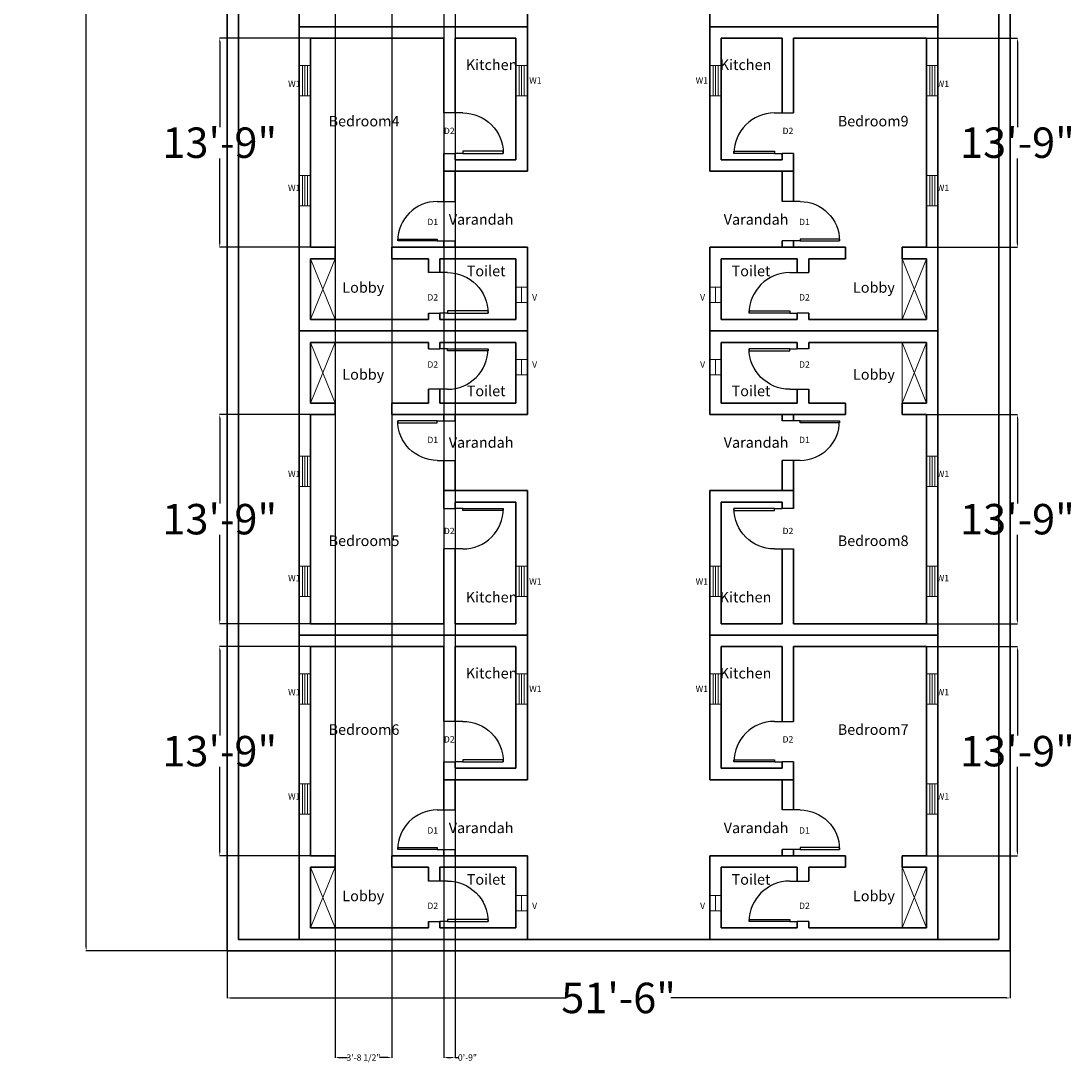
# Model space of a CAD drawing. Units: inches. Extents: x -205 to 674, y 63 to 1798.
# Tile 1 of 4: x -205 to 624, y 63 to 888. Entities that reach past the tile are written whole.
import ezdxf

# ---------------------------------------------------------------- set-up
doc = ezdxf.new("R2010")
doc.units = ezdxf.units.IN
doc.header["$MEASUREMENT"] = 0
doc.layers.get('0').update_dxf_attribs({"color": 70})
for name, color, linetype, lineweight in [('A-ANNO-DIMS', 240, 'Continuous', 18), ('A-ANNO-TEXT', 240, 'Continuous', 18), ('A-AREA-IDEN', 240, 'Continuous', 18), ('A-WALL', 70, 'Continuous', 35), ('A-WALL-SITE', 70, 'Continuous', 35), ('door1', 20, 'Continuous', 25), ('door2', 160, 'Continuous', 25), ('lobby', 241, 'Continuous', 18), ('ventilator1', 210, 'Continuous', 18), ('window1', 50, 'Continuous', 18)]:
    doc.layers.add(name, color=color, linetype=linetype, lineweight=lineweight)
doc.styles.get("Standard").update_dxf_attribs({"font": 'arial.ttf'})
doc.dimstyles.get("Standard").update_dxf_attribs({"dimtxt": 5, "dimasz": 3, "dimexe": 0.18, "dimexo": 0.0625, "dimgap": 0.09, "dimtad": 0, "dimtih": 1, "dimtoh": 1, "dimdec": 0, "dimzin": 0, "dimdsep": 46, "dimlunit": 3, "dimtxsty": 'Standard', "dimcen": 0.09, "dimadec": 0, "dimazin": 0, "dimtfac": 1, "dimtdec": 0, "dimtofl": 0, "dimtmove": 0, "dimatfit": 3, "dimfxl": 1, "dimtolj": 1, "dimtzin": 0, "dimarcsym": 0})

# ---------------------------------------------------------------- blocks, each defined once
blk = doc.blocks.new('*D8')
at = {"layer": 'A-ANNO-DIMS', "color": 0, "lineweight": -2, "transparency": 16777216}
for p, q in [((23.48, 874.3), (-48.36, 874.3)), ((-48.18, 871.3), (-48.18, 804.15)), ((-48.18, 712.3), (-48.18, 779.45)), ((23.48, 709.3), (-48.36, 709.3))]:
    blk.add_line(p, q, dxfattribs=at)
at = {"layer": 'A-ANNO-DIMS', "color": 0, "transparency": 16777216}
for points in [[(-48.68, 871.3), (-47.68, 871.3), (-48.18, 874.3)], [(-48.68, 712.3), (-47.68, 712.3), (-48.18, 709.3)]]:
    blk.add_solid(points, dxfattribs=at)
at = {"layer": 'Defpoints', "color": 0, "transparency": 16777216}
for p in [(-48.18, 874.3), (23.54, 874.3), (23.54, 709.3)]:
    blk.add_point(p, dxfattribs=at)
at = {"layer": 'A-ANNO-DIMS', "color": 0, "transparency": 16777216, "insert": (-48.18, 791.8), "char_height": 5, "attachment_point": 5}
blk.add_mtext('\\A1;{\\H4.8x;13\'-9"}', dxfattribs=at)
blk = doc.blocks.new('*U4')
for p, q in [((0, 0), (0, -6)), ((36, 0), (36, -6))]:
    blk.add_line(p, q)
blk.add_lwpolyline([(0, 0), (0, 36), (1.75, 36), (1.75, 0)], close=True)
blk.add_arc((0, 0), 36, 0, 90)
blk = doc.blocks.new('*U5')
for p, q in [((0, 0), (0, -6)), ((32, 0), (32, -6))]:
    blk.add_line(p, q)
blk.add_lwpolyline([(0, 0), (0, 32), (1.75, 32), (1.75, 0)], close=True)
blk.add_arc((0, 0), 32, 0, 90)
blk = doc.blocks.new('*D9')
at = {"layer": 'A-ANNO-DIMS', "color": 0, "lineweight": -2, "transparency": 16777216}
for p, q in [((23.48, 577.3), (-48.36, 577.3)), ((-48.18, 574.3), (-48.18, 507.15)), ((-48.18, 415.3), (-48.18, 482.45)), ((23.48, 412.3), (-48.36, 412.3))]:
    blk.add_line(p, q, dxfattribs=at)
at = {"layer": 'A-ANNO-DIMS', "color": 0, "transparency": 16777216}
for points in [[(-48.68, 574.3), (-47.68, 574.3), (-48.18, 577.3)], [(-48.68, 415.3), (-47.68, 415.3), (-48.18, 412.3)]]:
    blk.add_solid(points, dxfattribs=at)
at = {"layer": 'Defpoints', "color": 0, "transparency": 16777216}
for p in [(23.54, 577.3), (-48.18, 412.3), (23.54, 412.3)]:
    blk.add_point(p, dxfattribs=at)
at = {"layer": 'A-ANNO-DIMS', "color": 0, "transparency": 16777216, "insert": (-48.18, 494.8), "char_height": 5, "attachment_point": 5}
blk.add_mtext('\\A1;{\\H4.8x;13\'-9"}', dxfattribs=at)
blk = doc.blocks.new('*D10')
at = {"layer": 'A-ANNO-DIMS', "color": 0, "lineweight": -2, "transparency": 16777216}
for p, q in [((23.48, 394.3), (-48.36, 394.3)), ((-48.18, 391.3), (-48.18, 324.15)), ((-48.18, 232.3), (-48.18, 299.45)), ((23.48, 229.3), (-48.36, 229.3))]:
    blk.add_line(p, q, dxfattribs=at)
at = {"layer": 'A-ANNO-DIMS', "color": 0, "transparency": 16777216}
for points in [[(-48.68, 391.3), (-47.68, 391.3), (-48.18, 394.3)], [(-48.68, 232.3), (-47.68, 232.3), (-48.18, 229.3)]]:
    blk.add_solid(points, dxfattribs=at)
at = {"layer": 'Defpoints', "color": 0, "transparency": 16777216}
for p in [(-48.18, 394.3), (23.54, 394.3), (23.54, 229.3)]:
    blk.add_point(p, dxfattribs=at)
at = {"layer": 'A-ANNO-DIMS', "color": 0, "transparency": 16777216, "insert": (-48.18, 311.8), "char_height": 5, "attachment_point": 5}
blk.add_mtext('\\A1;{\\H4.8x;13\'-9"}', dxfattribs=at)
blk = doc.blocks.new('*D12')
at = {"layer": 'A-ANNO-DIMS', "color": 0, "lineweight": -2, "transparency": 16777216}
for p, q in [((509.6, 874.3), (581.44, 874.3)), ((581.26, 871.3), (581.26, 804.15)), ((581.26, 712.3), (581.26, 779.45)), ((509.6, 709.3), (581.44, 709.3))]:
    blk.add_line(p, q, dxfattribs=at)
at = {"layer": 'A-ANNO-DIMS', "color": 0, "transparency": 16777216}
for points in [[(580.76, 871.3), (581.76, 871.3), (581.26, 874.3)], [(580.76, 712.3), (581.76, 712.3), (581.26, 709.3)]]:
    blk.add_solid(points, dxfattribs=at)
at = {"layer": 'Defpoints', "color": 0, "transparency": 16777216}
for p in [(509.54, 874.3), (581.26, 874.3), (509.54, 709.3)]:
    blk.add_point(p, dxfattribs=at)
at = {"layer": 'A-ANNO-DIMS', "color": 0, "transparency": 16777216, "insert": (581.26, 791.8), "char_height": 5, "attachment_point": 5}
blk.add_mtext('\\A1;{\\H4.8x;13\'-9"}', dxfattribs=at)
blk = doc.blocks.new('*D13')
at = {"layer": 'A-ANNO-DIMS', "color": 0, "lineweight": -2, "transparency": 16777216}
for p, q in [((509.6, 577.3), (581.44, 577.3)), ((581.26, 574.3), (581.26, 507.15)), ((581.26, 415.3), (581.26, 482.45)), ((509.6, 412.3), (581.44, 412.3))]:
    blk.add_line(p, q, dxfattribs=at)
at = {"layer": 'A-ANNO-DIMS', "color": 0, "transparency": 16777216}
for points in [[(580.76, 574.3), (581.76, 574.3), (581.26, 577.3)], [(580.76, 415.3), (581.76, 415.3), (581.26, 412.3)]]:
    blk.add_solid(points, dxfattribs=at)
at = {"layer": 'Defpoints', "color": 0, "transparency": 16777216}
for p in [(509.54, 577.3), (509.54, 412.3), (581.26, 412.3)]:
    blk.add_point(p, dxfattribs=at)
at = {"layer": 'A-ANNO-DIMS', "color": 0, "transparency": 16777216, "insert": (581.26, 494.8), "char_height": 5, "attachment_point": 5}
blk.add_mtext('\\A1;{\\H4.8x;13\'-9"}', dxfattribs=at)
blk = doc.blocks.new('*D15')
at = {"layer": 'A-ANNO-DIMS', "color": 0, "lineweight": -2, "transparency": 16777216}
for p, q in [((509.6, 394.3), (581.44, 394.3)), ((581.26, 391.3), (581.26, 324.15)), ((581.26, 232.3), (581.26, 299.45)), ((509.6, 229.3), (581.44, 229.3))]:
    blk.add_line(p, q, dxfattribs=at)
at = {"layer": 'A-ANNO-DIMS', "color": 0, "transparency": 16777216}
for points in [[(580.76, 391.3), (581.76, 391.3), (581.26, 394.3)], [(580.76, 232.3), (581.76, 232.3), (581.26, 229.3)]]:
    blk.add_solid(points, dxfattribs=at)
at = {"layer": 'Defpoints', "color": 0, "transparency": 16777216}
for p in [(509.54, 394.3), (581.26, 394.3), (509.54, 229.3)]:
    blk.add_point(p, dxfattribs=at)
at = {"layer": 'A-ANNO-DIMS', "color": 0, "transparency": 16777216, "insert": (581.26, 311.8), "char_height": 5, "attachment_point": 5}
blk.add_mtext('\\A1;{\\H4.8x;13\'-9"}', dxfattribs=at)
blk = doc.blocks.new('*D18')
at = {"layer": 'A-ANNO-DIMS', "color": 0, "lineweight": -2, "transparency": 16777216}
for p, q in [((-42.52, 1660.3), (-153.74, 1660.3)), ((-153.56, 1657.3), (-153.56, 919.64)), ((-153.56, 157.3), (-153.56, 894.96)), ((-42.52, 154.3), (-153.74, 154.3))]:
    blk.add_line(p, q, dxfattribs=at)
at = {"layer": 'A-ANNO-DIMS', "color": 0, "transparency": 16777216}
for points in [[(-154.06, 1657.3), (-153.06, 1657.3), (-153.56, 1660.3)], [(-154.06, 157.3), (-153.06, 157.3), (-153.56, 154.3)]]:
    blk.add_solid(points, dxfattribs=at)
at = {"layer": 'Defpoints', "color": 0, "transparency": 16777216}
for p in [(-42.46, 1660.3), (-153.56, 154.3), (-42.46, 154.3)]:
    blk.add_point(p, dxfattribs=at)
at = {"layer": 'A-ANNO-DIMS', "color": 0, "transparency": 16777216, "insert": (-153.56, 907.3), "char_height": 5, "attachment_point": 5}
blk.add_mtext('\\A1;{\\H4.8x;125\'-6"}', dxfattribs=at)
blk = doc.blocks.new('*D19')
at = {"layer": 'A-ANNO-DIMS', "color": 0, "lineweight": -2, "transparency": 16777216}
for p, q in [((-42.46, 154.24), (-42.46, 116.92)), ((575.54, 154.24), (575.54, 116.92)), ((-39.46, 117.1), (225.23, 117.1)), ((572.54, 117.1), (307.85, 117.1))]:
    blk.add_line(p, q, dxfattribs=at)
at = {"layer": 'A-ANNO-DIMS', "color": 0, "transparency": 16777216}
for points in [[(-39.46, 117.6), (-39.46, 116.6), (-42.46, 117.1)], [(572.54, 117.6), (572.54, 116.6), (575.54, 117.1)]]:
    blk.add_solid(points, dxfattribs=at)
at = {"layer": 'Defpoints', "color": 0, "transparency": 16777216}
for p in [(-42.46, 154.3), (575.54, 154.3), (575.54, 117.1)]:
    blk.add_point(p, dxfattribs=at)
at = {"layer": 'A-ANNO-DIMS', "color": 0, "transparency": 16777216, "insert": (266.54, 117.1), "char_height": 5, "attachment_point": 5}
blk.add_mtext('\\A1;{\\H4.8x;51\'-6"}', dxfattribs=at)
blk = doc.blocks.new('WIN-W1-24IN')
for p, q in [((2.5, 24), (2.5, 0)), ((4.5, 24), (4.5, 0)), ((6.5, 24), (6.5, 0))]:
    blk.add_line(p, q)
blk.add_lwpolyline([(0, 24), (9, 24), (9, 0), (0, 0)], close=True)
blk = doc.blocks.new('VENT-V-12IN')
blk.add_line((4.5, 12), (4.5, 0))
blk.add_lwpolyline([(9, 0), (0, 0), (0, 12), (9, 12)], close=True)
blk = doc.blocks.new('LOBBY-RECESS')
for p, q in [((0, 48), (19.36, 0)), ((0, 0), (19.36, 48)), ((19.36, 48), (19.36, 0))]:
    blk.add_line(p, q)
blk = doc.blocks.new('*D40')
at = {"layer": 'A-ANNO-DIMS', "color": 0, "lineweight": -2, "transparency": 16777216}
for p, q in [((128.54, 1372.24), (128.54, 69.92)), ((137.54, 1372.24), (137.54, 69.92)), ((131.54, 70.1), (134.54, 70.1)), ((137.54, 70.1), (140.54, 70.1))]:
    blk.add_line(p, q, dxfattribs=at)
at = {"layer": 'A-ANNO-DIMS', "color": 0, "transparency": 16777216}
for points in [[(131.54, 70.6), (131.54, 69.6), (128.54, 70.1)], [(134.54, 70.6), (134.54, 69.6), (137.54, 70.1)]]:
    blk.add_solid(points, dxfattribs=at)
at = {"layer": 'Defpoints', "color": 0, "transparency": 16777216}
for p in [(128.54, 1372.3), (137.54, 1372.3), (137.54, 70.1)]:
    blk.add_point(p, dxfattribs=at)
at = {"layer": 'A-ANNO-DIMS', "color": 0, "transparency": 16777216, "insert": (147.28, 70.1), "char_height": 5, "attachment_point": 5}
blk.add_mtext('\\A1;0\'-9"', dxfattribs=at)
blk = doc.blocks.new('*D47')
at = {"layer": 'A-ANNO-DIMS', "color": 0, "lineweight": -2, "transparency": 16777216}
for p, q in [((42.9, 1546.24), (42.9, 69.92)), ((87.49, 1546.24), (87.49, 69.92)), ((45.9, 70.1), (52.64, 70.1)), ((84.49, 70.1), (77.76, 70.1))]:
    blk.add_line(p, q, dxfattribs=at)
at = {"layer": 'A-ANNO-DIMS', "color": 0, "transparency": 16777216}
for points in [[(45.9, 70.6), (45.9, 69.6), (42.9, 70.1)], [(84.49, 70.6), (84.49, 69.6), (87.49, 70.1)]]:
    blk.add_solid(points, dxfattribs=at)
at = {"layer": 'Defpoints', "color": 0, "transparency": 16777216}
for p in [(42.9, 1546.3), (87.49, 1546.3), (87.49, 70.1)]:
    blk.add_point(p, dxfattribs=at)
at = {"layer": 'A-ANNO-DIMS', "color": 0, "transparency": 16777216, "insert": (65.2, 70.1), "char_height": 5, "attachment_point": 5}
blk.add_mtext('\\A1;3\'-8 1/2"', dxfattribs=at)

msp = doc.modelspace()

# ---------------------------------------------------------------- linework, layer by layer
at = {"layer": 'A-WALL'}
for p, q in [((14.54, 883.3), (14.54, 1123.3)), ((518.54, 883.3), (518.54, 1123.3)), ((194.54, 997.3), (194.54, 883.3)), ((338.54, 997.3), (338.54, 883.3)), ((14.54, 883.3), (194.54, 883.3)), ((14.54, 883.3), (14.54, 643.3)), ((14.54, 883.3), (194.54, 883.3)), ((194.54, 769.3), (194.54, 883.3)), ((518.54, 883.3), (338.54, 883.3)), ((338.54, 769.3), (338.54, 883.3)), ((518.54, 883.3), (338.54, 883.3)), ((518.54, 883.3), (518.54, 643.3)), ((128.54, 874.3), (23.54, 874.3)), ((23.54, 874.3), (23.54, 709.3)), ((128.54, 815.3), (128.54, 874.3)), ((137.54, 815.3), (137.54, 874.3)), ((185.54, 874.3), (137.54, 874.3)), ((137.54, 815.3), (137.54, 874.3)), ((185.54, 778.3), (185.54, 874.3)), ((347.54, 778.3), (347.54, 874.3)), ((347.54, 874.3), (395.54, 874.3)), ((395.54, 815.3), (395.54, 874.3)), ((395.54, 815.3), (395.54, 874.3)), ((404.54, 815.3), (404.54, 874.3)), ((404.54, 874.3), (509.54, 874.3)), ((509.54, 874.3), (509.54, 709.3)), ((128.54, 745.41), (128.54, 783.3)), ((128.54, 783.3), (128.54, 778.3)), ((137.54, 778.3), (137.54, 783.3)), ((137.54, 778.3), (137.54, 783.3)), ((395.54, 778.3), (395.54, 783.3)), ((395.54, 778.3), (395.54, 783.3)), ((404.54, 745.41), (404.54, 783.3)), ((404.54, 783.3), (404.54, 778.3)), ((185.54, 778.3), (137.54, 778.3)), ((347.54, 778.3), (395.54, 778.3)), ((194.54, 769.3), (128.54, 769.3)), ((137.54, 745.41), (137.54, 769.3)), ((338.54, 769.3), (404.54, 769.3)), ((395.54, 745.41), (395.54, 769.3)), ((128.54, 709.3), (128.54, 714.3)), ((137.54, 709.3), (137.54, 714.3)), ((137.55, 709.3), (137.55, 714.2)), ((395.54, 709.3), (395.54, 714.3)), ((395.54, 709.3), (395.54, 714.2)), ((404.54, 709.3), (404.54, 714.3)), ((23.54, 709.3), (42.9, 709.3)), ((42.9, 700.3), (42.9, 709.3)), ((42.9, 709.3), (42.9, 709.3)), ((87.49, 709.3), (194.54, 709.3)), ((87.49, 700.3), (87.49, 709.3)), ((87.49, 709.3), (87.49, 709.3)), ((194.54, 643.3), (194.54, 709.3)), ((338.54, 643.3), (338.54, 709.3)), ((445.59, 709.3), (338.54, 709.3)), ((445.59, 700.3), (445.59, 709.3)), ((445.59, 709.3), (445.59, 709.3)), ((509.54, 709.3), (490.18, 709.3)), ((490.18, 700.3), (490.18, 709.3)), ((490.18, 709.3), (490.18, 709.3)), ((23.54, 700.3), (42.9, 700.3)), ((23.54, 700.3), (23.54, 652.3)), ((87.49, 700.3), (116.54, 700.3)), ((116.54, 689.3), (116.54, 700.3)), ((125.54, 700.3), (185.54, 700.3)), ((125.54, 689.3), (125.54, 700.3)), ((185.54, 652.3), (185.54, 700.3)), ((407.54, 700.3), (347.54, 700.3)), ((347.54, 652.3), (347.54, 700.3)), ((407.54, 689.3), (407.54, 700.3)), ((445.59, 700.3), (416.54, 700.3)), ((416.54, 689.3), (416.54, 700.3)), ((509.54, 700.3), (490.18, 700.3)), ((509.54, 700.3), (509.54, 652.3)), ((116.54, 652.3), (116.54, 657.3)), ((116.54, 657.3), (116.54, 652.3)), ((125.54, 652.3), (125.54, 657.3)), ((125.54, 652.3), (125.54, 657.3)), ((407.54, 652.3), (407.54, 657.3)), ((407.54, 652.3), (407.54, 657.3)), ((416.54, 652.3), (416.54, 657.3)), ((416.54, 657.3), (416.54, 652.3)), ((23.54, 652.3), (116.54, 652.3)), ((125.54, 652.3), (185.54, 652.3)), ((407.54, 652.3), (347.54, 652.3)), ((509.54, 652.3), (416.54, 652.3)), ((14.54, 643.3), (194.54, 643.3)), ((14.54, 643.3), (194.54, 643.3)), ((14.54, 643.3), (194.54, 643.3)), ((14.54, 643.3), (194.54, 643.3)), ((14.54, 403.3), (14.54, 643.3)), ((194.54, 643.3), (194.54, 577.3)), ((518.54, 643.3), (338.54, 643.3)), ((518.54, 643.3), (338.54, 643.3)), ((518.54, 643.3), (338.54, 643.3)), ((518.54, 643.3), (338.54, 643.3)), ((338.54, 643.3), (338.54, 577.3)), ((518.54, 403.3), (518.54, 643.3)), ((23.54, 634.3), (116.54, 634.3)), ((23.54, 586.3), (23.54, 634.3)), ((116.54, 634.3), (116.54, 629.3)), ((116.54, 629.3), (116.54, 634.3)), ((125.54, 634.3), (185.54, 634.3)), ((125.54, 634.3), (125.54, 629.3)), ((125.54, 634.3), (125.54, 629.3)), ((185.54, 634.3), (185.54, 586.3)), ((407.54, 634.3), (347.54, 634.3)), ((347.54, 634.3), (347.54, 586.3)), ((407.54, 634.3), (407.54, 629.3)), ((407.54, 634.3), (407.54, 629.3)), ((509.54, 634.3), (416.54, 634.3)), ((416.54, 634.3), (416.54, 629.3)), ((416.54, 629.3), (416.54, 634.3)), ((509.54, 586.3), (509.54, 634.3)), ((116.54, 597.3), (116.54, 586.3)), ((125.54, 597.3), (125.54, 586.3)), ((407.54, 597.3), (407.54, 586.3)), ((416.54, 597.3), (416.54, 586.3)), ((23.54, 586.3), (42.9, 586.3)), ((42.9, 586.3), (42.9, 577.3)), ((87.49, 586.3), (116.54, 586.3)), ((87.49, 586.3), (87.49, 577.3)), ((125.54, 586.3), (185.54, 586.3)), ((407.54, 586.3), (347.54, 586.3)), ((445.59, 586.3), (416.54, 586.3)), ((445.59, 586.3), (445.59, 577.3)), ((509.54, 586.3), (490.18, 586.3)), ((490.18, 586.3), (490.18, 577.3)), ((23.54, 577.3), (42.9, 577.3)), ((23.54, 412.3), (23.54, 577.3)), ((42.9, 577.3), (42.9, 577.3)), ((87.49, 577.3), (194.54, 577.3)), ((87.49, 577.3), (87.49, 577.3)), ((128.54, 577.3), (128.54, 572.3)), ((137.54, 577.3), (137.54, 572.3)), ((137.55, 577.29), (137.55, 572.4)), ((445.59, 577.3), (338.54, 577.3)), ((395.54, 577.3), (395.54, 572.3)), ((395.54, 577.29), (395.54, 572.4)), ((404.54, 577.3), (404.54, 572.3)), ((445.59, 577.3), (445.59, 577.3)), ((509.54, 577.3), (490.18, 577.3)), ((490.18, 577.3), (490.18, 577.3)), ((509.54, 412.3), (509.54, 577.3)), ((128.54, 541.19), (128.54, 503.3)), ((137.54, 541.19), (137.54, 517.3)), ((395.54, 541.19), (395.54, 517.3)), ((404.54, 541.19), (404.54, 503.3)), ((194.54, 517.3), (128.54, 517.3)), ((194.54, 517.3), (194.54, 403.3)), ((338.54, 517.3), (338.54, 403.3)), ((338.54, 517.3), (404.54, 517.3)), ((128.54, 503.3), (128.54, 508.3)), ((137.54, 508.3), (137.54, 503.3)), ((185.54, 508.3), (137.54, 508.3)), ((137.54, 508.3), (137.54, 503.3)), ((185.54, 508.3), (185.54, 412.3)), ((347.54, 508.3), (347.54, 412.3)), ((347.54, 508.3), (395.54, 508.3)), ((395.54, 508.3), (395.54, 503.3)), ((395.54, 508.3), (395.54, 503.3)), ((404.54, 503.3), (404.54, 508.3)), ((128.54, 471.3), (128.54, 412.3)), ((137.54, 471.3), (137.54, 412.3)), ((137.54, 471.3), (137.54, 412.3)), ((395.54, 471.3), (395.54, 412.3)), ((395.54, 471.3), (395.54, 412.3)), ((404.54, 471.3), (404.54, 412.3)), ((128.54, 412.3), (23.54, 412.3)), ((185.54, 412.3), (137.54, 412.3)), ((347.54, 412.3), (395.54, 412.3)), ((404.54, 412.3), (509.54, 412.3)), ((14.54, 403.3), (194.54, 403.3)), ((14.54, 403.3), (14.54, 163.3)), ((14.54, 403.3), (194.54, 403.3)), ((194.54, 289.3), (194.54, 403.3)), ((518.54, 403.3), (338.54, 403.3)), ((338.54, 289.3), (338.54, 403.3)), ((518.54, 403.3), (338.54, 403.3)), ((518.54, 403.3), (518.54, 163.3)), ((128.54, 394.3), (23.54, 394.3)), ((23.54, 394.3), (23.54, 229.3)), ((128.54, 335.3), (128.54, 394.3)), ((137.54, 335.3), (137.54, 394.3)), ((185.54, 394.3), (137.54, 394.3)), ((137.54, 335.3), (137.54, 394.3)), ((185.54, 298.3), (185.54, 394.3)), ((347.54, 298.3), (347.54, 394.3)), ((347.54, 394.3), (395.54, 394.3)), ((395.54, 335.3), (395.54, 394.3)), ((395.54, 335.3), (395.54, 394.3)), ((404.54, 335.3), (404.54, 394.3)), ((404.54, 394.3), (509.54, 394.3)), ((509.54, 394.3), (509.54, 229.3)), ((128.54, 265.41), (128.54, 303.3)), ((128.54, 303.3), (128.54, 298.3)), ((137.54, 298.3), (137.54, 303.3)), ((137.54, 298.3), (137.54, 303.3)), ((185.54, 298.3), (137.54, 298.3)), ((347.54, 298.3), (395.54, 298.3)), ((395.54, 298.3), (395.54, 303.3)), ((395.54, 298.3), (395.54, 303.3)), ((404.54, 265.41), (404.54, 303.3)), ((404.54, 303.3), (404.54, 298.3)), ((194.54, 289.3), (128.54, 289.3)), ((137.54, 265.41), (137.54, 289.3)), ((338.54, 289.3), (404.54, 289.3)), ((395.54, 265.41), (395.54, 289.3)), ((128.54, 229.3), (128.54, 234.3)), ((137.54, 229.3), (137.54, 234.3)), ((137.55, 229.3), (137.55, 234.2)), ((395.54, 229.3), (395.54, 234.3)), ((395.54, 229.3), (395.54, 234.2)), ((404.54, 229.3), (404.54, 234.3)), ((23.54, 229.3), (42.9, 229.3)), ((42.9, 220.3), (42.9, 229.3)), ((42.9, 229.3), (42.9, 229.3)), ((87.49, 229.3), (194.54, 229.3)), ((87.49, 220.3), (87.49, 229.3)), ((87.49, 229.3), (87.49, 229.3)), ((194.54, 163.3), (194.54, 229.3)), ((338.54, 163.3), (338.54, 229.3)), ((445.59, 229.3), (338.54, 229.3)), ((445.59, 220.3), (445.59, 229.3)), ((445.59, 229.3), (445.59, 229.3)), ((509.54, 229.3), (490.18, 229.3)), ((490.18, 220.3), (490.18, 229.3)), ((490.18, 229.3), (490.18, 229.3)), ((23.54, 220.3), (42.9, 220.3)), ((23.54, 220.3), (23.54, 172.3)), ((87.49, 220.3), (116.54, 220.3)), ((116.54, 209.3), (116.54, 220.3)), ((125.54, 220.3), (185.54, 220.3)), ((125.54, 209.3), (125.54, 220.3)), ((185.54, 172.3), (185.54, 220.3)), ((407.54, 220.3), (347.54, 220.3)), ((347.54, 172.3), (347.54, 220.3)), ((407.54, 209.3), (407.54, 220.3)), ((445.59, 220.3), (416.54, 220.3)), ((416.54, 209.3), (416.54, 220.3)), ((509.54, 220.3), (490.18, 220.3)), ((509.54, 220.3), (509.54, 172.3)), ((116.54, 172.3), (116.54, 177.3)), ((116.54, 177.3), (116.54, 172.3)), ((125.54, 172.3), (125.54, 177.3)), ((125.54, 172.3), (125.54, 177.3)), ((407.54, 172.3), (407.54, 177.3)), ((407.54, 172.3), (407.54, 177.3)), ((416.54, 172.3), (416.54, 177.3)), ((416.54, 177.3), (416.54, 172.3)), ((23.54, 172.3), (116.54, 172.3)), ((125.54, 172.3), (185.54, 172.3)), ((407.54, 172.3), (347.54, 172.3)), ((509.54, 172.3), (416.54, 172.3))]:
    msp.add_line(p, q, dxfattribs=at)
at = {"layer": 'A-WALL-SITE'}
for p, q in [((-33.46, 403.3), (-33.46, 163.3)), ((566.54, 403.3), (566.54, 163.3))]:
    msp.add_line(p, q, dxfattribs=at)
for points in [[(575.54, 154.3), (575.54, 1660.3), (266.54, 1660.3), (-42.46, 1660.3), (-42.46, 154.3), (266.54, 154.3)], [(566.54, 163.3), (566.54, 1651.3), (266.54, 1651.3), (-33.46, 1651.3), (-33.46, 163.3), (266.54, 163.3)]]:
    msp.add_lwpolyline(points, close=True, dxfattribs=at)
at = {"layer": 'door1'}
for p, q in [((128.54, 745.41), (137.54, 745.41)), ((404.54, 745.41), (395.54, 745.41)), ((128.54, 714.3), (137.54, 714.3)), ((404.54, 714.3), (395.54, 714.3)), ((128.54, 572.3), (137.54, 572.3)), ((404.54, 572.3), (395.54, 572.3)), ((128.54, 541.19), (137.54, 541.19)), ((404.54, 541.19), (395.54, 541.19)), ((128.54, 265.41), (137.54, 265.41)), ((404.54, 265.41), (395.54, 265.41)), ((128.54, 234.3), (137.54, 234.3)), ((404.54, 234.3), (395.54, 234.3))]:
    msp.add_line(p, q, dxfattribs=at)
at = {"layer": 'door2'}
for p, q in [((137.54, 815.3), (128.54, 815.3)), ((395.54, 815.3), (404.54, 815.3)), ((128.54, 783.3), (137.54, 783.3)), ((404.54, 783.3), (395.54, 783.3)), ((125.54, 689.3), (116.54, 689.3)), ((407.54, 689.3), (416.54, 689.3)), ((116.54, 657.3), (125.54, 657.3)), ((416.54, 657.3), (407.54, 657.3)), ((116.54, 629.3), (125.54, 629.3)), ((416.54, 629.3), (407.54, 629.3)), ((125.54, 597.3), (116.54, 597.3)), ((407.54, 597.3), (416.54, 597.3)), ((128.54, 503.3), (137.54, 503.3)), ((404.54, 503.3), (395.54, 503.3)), ((137.54, 471.3), (128.54, 471.3)), ((395.54, 471.3), (404.54, 471.3)), ((137.54, 335.3), (128.54, 335.3)), ((395.54, 335.3), (404.54, 335.3)), ((128.54, 303.3), (137.54, 303.3)), ((404.54, 303.3), (395.54, 303.3)), ((125.54, 209.3), (116.54, 209.3)), ((407.54, 209.3), (416.54, 209.3)), ((116.54, 177.3), (125.54, 177.3)), ((416.54, 177.3), (407.54, 177.3))]:
    msp.add_line(p, q, dxfattribs=at)

# ---------------------------------------------------------------- block references
at = {"layer": 'door1', "yscale": 0.8640557789234337, "zscale": 0.8640557789234337}
for p, xscale, rotation in [((123.36, 714.3), 0.8640557789234337, 90.00000000000003), ((409.73, 714.3), -0.8640557789234337, 270), ((123.36, 572.3), -0.8640557789234337, 90), ((409.73, 572.3), 0.8640557789234337, 270), ((123.36, 234.3), 0.8640557789234337, 90.00000000000003), ((409.73, 234.3), -0.8640557789234337, 270)]:
    msp.add_blockref('*U4', p, dxfattribs=dict(at, xscale=xscale, rotation=rotation))
at = {"layer": 'door2', "xscale": -1}
for p, rotation in [((143.54, 783.3), 270), ((131.54, 657.3), 270), ((401.54, 629.3), 90), ((389.54, 503.3), 90), ((143.54, 303.3), 270), ((131.54, 177.3), 270)]:
    msp.add_blockref('*U5', p, dxfattribs=dict(at, rotation=rotation))
at = {"layer": 'door2'}
for p, rotation in [((389.54, 783.3), 90.00000000000003), ((401.54, 657.3), 90.00000000000003), ((131.54, 629.3), 270), ((143.54, 503.3), 270), ((389.54, 303.3), 90.00000000000003), ((401.54, 177.3), 90.00000000000003)]:
    msp.add_blockref('*U5', p, dxfattribs=dict(at, rotation=rotation))
at = {"layer": 'lobby'}
for p in [(23.54, 652.3), (23.54, 586.3), (23.54, 172.3)]:
    msp.add_blockref('LOBBY-RECESS', p, dxfattribs=at)
at = {"layer": 'lobby', "rotation": 180}
for p in [(509.54, 700.3), (509.54, 634.3), (509.54, 220.3)]:
    msp.add_blockref('LOBBY-RECESS', p, dxfattribs=at)
at = {"layer": 'ventilator1', "extrusion": (0, 0, -1), "zscale": -1, "rotation": 180}
for p in [(-185.54, 677.85), (-185.54, 197.85)]:
    msp.add_blockref('VENT-V-12IN', p, dxfattribs=at)
at = {"layer": 'ventilator1', "rotation": 180}
for p in [(347.54, 677.85), (347.54, 197.85)]:
    msp.add_blockref('VENT-V-12IN', p, dxfattribs=at)
at = {"layer": 'ventilator1'}
msp.add_blockref('VENT-V-12IN', (185.54, 608.75), dxfattribs=at)
at = {"layer": 'ventilator1', "extrusion": (0, 0, -1), "zscale": -1}
msp.add_blockref('VENT-V-12IN', (-347.54, 608.75), dxfattribs=at)
at = {"layer": 'window1', "extrusion": (0, 0, -1), "zscale": -1, "rotation": 180}
for p in [(-14.54, 852.79), (-185.54, 852.79), (-14.54, 766.03), (-14.54, 372.79), (-185.54, 372.79), (-14.54, 286.03)]:
    msp.add_blockref('WIN-W1-24IN', p, dxfattribs=at)
at = {"layer": 'window1', "rotation": 180}
for p in [(347.54, 852.79), (518.54, 852.79), (518.54, 766.03), (347.54, 372.79), (518.54, 372.79), (518.54, 286.03)]:
    msp.add_blockref('WIN-W1-24IN', p, dxfattribs=at)
at = {"layer": 'window1'}
for p in [(14.54, 520.57), (14.54, 433.81), (185.54, 433.81)]:
    msp.add_blockref('WIN-W1-24IN', p, dxfattribs=at)
at = {"layer": 'window1', "extrusion": (0, 0, -1), "zscale": -1}
for p in [(-518.54, 520.57), (-347.54, 433.81), (-518.54, 433.81)]:
    msp.add_blockref('WIN-W1-24IN', p, dxfattribs=at)

# ---------------------------------------------------------------- texts
at = {"layer": 'A-ANNO-TEXT', "char_height": 5}
for s, insert, attachment_point in [('W1', (5.74, 835.77), 7), ('W1', (195.97, 838.49), 7), ('W1', (337.12, 838.49), 9), ('W1', (527.34, 835.77), 9), ('D2', (128.68, 798.61), 7), ('D2', (404.41, 798.61), 9), ('W1', (5.68, 753.64), 7), ('W1', (527.4, 753.64), 9), ('D1', (115.64, 726.76), 7), ('D1', (417.45, 726.76), 9), ('D2', (115.64, 667.31), 7), ('V', (198.3, 667.31), 7), ('V', (334.78, 667.31), 9), ('D2', (417.45, 667.31), 9), ('D2', (115.64, 619.29), 1), ('V', (198.3, 619.29), 1), ('V', (334.78, 619.29), 3), ('D2', (417.45, 619.29), 3), ('D1', (115.64, 559.84), 1), ('D1', (417.45, 559.84), 3), ('W1', (5.68, 532.96), 1), ('W1', (527.4, 532.96), 3), ('D2', (128.68, 487.99), 1), ('D2', (404.41, 487.99), 3), ('W1', (5.74, 450.83), 1), ('W1', (195.97, 448.11), 1), ('W1', (337.12, 448.11), 3), ('W1', (527.34, 450.83), 3), ('W1', (5.74, 355.77), 7), ('W1', (195.97, 358.49), 7), ('W1', (337.12, 358.49), 9), ('W1', (527.34, 355.77), 9), ('D2', (128.68, 318.61), 7), ('D2', (404.41, 318.61), 9), ('W1', (5.68, 273.64), 7), ('W1', (527.4, 273.64), 9), ('D1', (115.64, 246.76), 7), ('D1', (417.45, 246.76), 9), ('D2', (115.64, 187.31), 7), ('V', (198.3, 187.31), 7), ('V', (334.78, 187.31), 9), ('D2', (417.45, 187.31), 9)]:
    msp.add_mtext_dynamic_manual_height_columns(s, width=13.5017, gutter_width=1, heights=[0], dxfattribs=dict(at, insert=insert, attachment_point=attachment_point))
at = {"layer": 'A-AREA-IDEN', "char_height": 8.34}
for s, insert, attachment_point in [('Kitchen', (145.99, 849.12), 7), ('Kitchen', (387.1, 849.12), 9), ('Bedroom4', (37.73, 804.65), 7), ('Bedroom9', (495.36, 804.65), 9), ('Varandah', (132.52, 727.11), 7), ('Varandah', (400.56, 727.11), 9), ('Toilet', (146.71, 686.44), 7), ('Toilet', (386.37, 686.44), 9), ('Lobby', (48.54, 673.43), 7), ('Lobby', (484.55, 673.43), 9), ('Lobby', (48.54, 613.17), 1), ('Lobby', (484.55, 613.17), 3), ('Toilet', (146.71, 600.16), 1), ('Toilet', (386.37, 600.16), 3), ('Varandah', (132.52, 559.49), 1), ('Varandah', (400.56, 559.49), 3), ('Bedroom5', (37.73, 481.95), 1), ('Bedroom8', (495.36, 481.95), 3), ('Kitchen', (145.99, 437.47), 1), ('Kitchen', (387.1, 437.47), 3), ('Kitchen', (145.99, 369.12), 7), ('Kitchen', (387.1, 369.12), 9), ('Bedroom6', (37.73, 324.65), 7), ('Bedroom7', (495.36, 324.65), 9), ('Varandah', (132.52, 247.11), 7), ('Varandah', (400.56, 247.11), 9), ('Toilet', (146.71, 206.44), 7), ('Toilet', (386.37, 206.44), 9), ('Lobby', (48.54, 193.43), 7), ('Lobby', (484.55, 193.43), 9)]:
    msp.add_mtext_dynamic_manual_height_columns(s, width=37.3149, gutter_width=1.67, heights=[0], dxfattribs=dict(at, insert=insert, attachment_point=attachment_point))

# ---------------------------------------------------------------- dimensions: what is measured, and where the dimension line sits
at = {"layer": 'A-ANNO-DIMS'}
for base, p1, p2, angle, picture, middle in [((-153.56, 154.3), (-42.46, 1660.3), (-42.46, 154.3), 90, '*D18', (-153.56, 907.3)), ((-48.18, 874.3), (23.54, 709.3), (23.54, 874.3), 270, '*D8', (-48.18, 791.8)), ((581.26, 874.3), (509.54, 709.3), (509.54, 874.3), 270, '*D12', (581.26, 791.8)), ((-48.18, 412.3), (23.54, 577.3), (23.54, 412.3), 90, '*D9', (-48.18, 494.8)), ((581.26, 412.3), (509.54, 577.3), (509.54, 412.3), 90, '*D13', (581.26, 494.8)), ((-48.18, 394.3), (23.54, 229.3), (23.54, 394.3), 270, '*D10', (-48.18, 311.8)), ((581.26, 394.3), (509.54, 229.3), (509.54, 394.3), 270, '*D15', (581.26, 311.8))]:
    dim = msp.add_linear_dim(base=base, p1=p1, p2=p2, angle=angle, text='{\\H4.8x;<>}', dimstyle='Standard', override={"dimclrd": 0, "dimclre": 0, "dimclrt": 0}, dxfattribs=at)
    dim.commit()
    dim.dimension.update_dxf_attribs({"geometry": picture, "text_midpoint": middle})
for base, p1, p2, picture, middle in [((87.49, 70.1), (42.9, 1546.3), (87.49, 1546.3), '*D47', (65.2, 70.1)), ((137.54, 70.1), (128.54, 1372.3), (137.54, 1372.3), '*D40', (147.28, 70.1))]:
    dim = msp.add_linear_dim(base=base, p1=p1, p2=p2, dimstyle='Standard', override={"dimdec": 1, "dimlfac": 1, "dimrnd": 0, "dimzin": 1, "dimdsep": 46, "dimlunit": 4, "dimfrac": 2}, dxfattribs=at)
    dim.commit()
    dim.dimension.update_dxf_attribs({"geometry": picture, "text_midpoint": middle})
dim = msp.add_linear_dim(base=(575.54, 117.1), p1=(-42.46, 154.3), p2=(575.54, 154.3), text='{\\H4.8x;<>}', dimstyle='Standard', override={"dimclrd": 0, "dimclre": 0, "dimclrt": 0}, dxfattribs=at)
dim.commit()
dim.dimension.update_dxf_attribs({"geometry": '*D19', "text_midpoint": (266.54, 117.1)})

doc.saveas('drawing.dxf')
